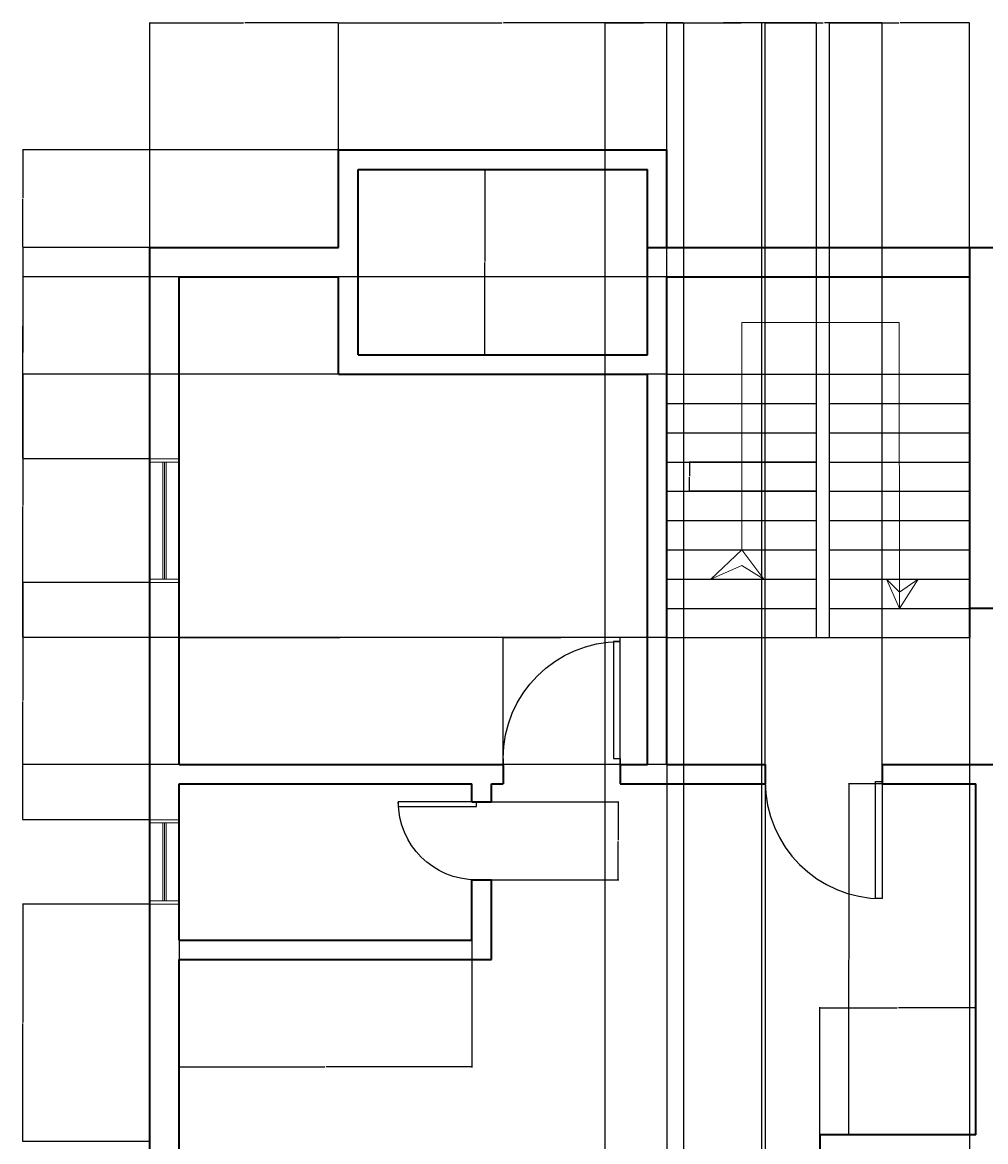
# Model space of a CAD drawing. Units: inches. Extents: x -7288 to -6705, y 7169 to 8028.
# Tile 4 of 5: x -7288 to -6992, y 7684 to 8028. Entities that reach past the tile are written whole.
import ezdxf

# ---------------------------------------------------------------- set-up
doc = ezdxf.new("R2010")
doc.units = ezdxf.units.IN
for name, color, linetype, lineweight in [('A-ANNO-DIMS', 2, 'Continuous', 18), ('A-ANNO-SYMB', 7, 'Continuous', 18), ('A-DOOR', 3, 'Continuous', 25), ('A-FLOR-STRS', 1, 'Continuous', 25), ('A-GLAZ', 2, 'Continuous', 18), ('A-WALL', 1, 'Continuous', 35)]:
    doc.layers.add(name, color=color, linetype=linetype, lineweight=lineweight)
doc.styles.get("Standard").update_dxf_attribs({"font": 'arial.ttf'})
doc.dimstyles.get("Standard").update_dxf_attribs({"dimtxt": 0.18, "dimasz": 0.18, "dimexe": 0.18, "dimexo": 0.0625, "dimgap": 0.09, "dimtad": 0, "dimtih": 1, "dimtoh": 1, "dimdec": 4, "dimzin": 0, "dimdsep": 46, "dimtxsty": 'Standard', "dimcen": 0.09, "dimadec": 0, "dimazin": 0, "dimtfac": 1, "dimtdec": 4, "dimtofl": 0, "dimtmove": 0, "dimatfit": 3, "dimfxl": 1, "dimtolj": 1, "dimtzin": 0, "dimarcsym": 0})

# ---------------------------------------------------------------- blocks, each defined once
blk = doc.blocks.new('*U8')
for p, q in [((0, 0), (0, -100)), ((750, 0), (750, -100))]:
    blk.add_line(p, q)
blk.add_lwpolyline([(0, 0), (0, 750), (43.75, 750), (43.75, 0)], close=True)
blk.add_arc((0, 0), 750, 0, 90)
blk = doc.blocks.new('WIN-36IN-WALL9')
for p, q in [((0, 38), (9, 38)), ((0, 37), (9, 37)), ((4, 1), (4, 37)), ((4.5, 1), (4.5, 37)), ((5, 1), (5, 37)), ((0, 1), (9, 1)), ((0, 0), (9, 0))]:
    blk.add_line(p, q)
blk = doc.blocks.new('WIN-24IN-WALL9')
for p, q in [((0, 26), (9, 26)), ((0, 25), (9, 25)), ((4, 1), (4, 25)), ((4.5, 1), (4.5, 25)), ((5, 1), (5, 25)), ((0, 1), (9, 1)), ((0, 0), (9, 0))]:
    blk.add_line(p, q)
blk = doc.blocks.new('*D95')
at = {"layer": 'A-ANNO-DIMS', "color": 0, "lineweight": -2, "transparency": 16777216}
for p, q in [((-7248.84, 7958.59), (-7248.84, 8027.74)), ((-7248.66, 8027.56), (-7220.06, 8027.56)), ((-7191.02, 8027.56), (-7219.62, 8027.56)), ((-7190.84, 7988.59), (-7190.84, 8027.74))]:
    blk.add_line(p, q, dxfattribs=at)
at = {"layer": 'A-ANNO-DIMS', "color": 0, "transparency": 16777216}
for points in [[(-7248.66, 8027.59), (-7248.66, 8027.53), (-7248.84, 8027.56)], [(-7191.02, 8027.59), (-7191.02, 8027.53), (-7190.84, 8027.56)]]:
    blk.add_solid(points, dxfattribs=at)
at = {"layer": 'Defpoints', "color": 0, "transparency": 16777216}
for p in [(-7190.84, 8027.56), (-7190.84, 7988.53), (-7248.84, 7958.53)]:
    blk.add_point(p, dxfattribs=at)
at = {"layer": 'A-ANNO-DIMS', "color": 0, "transparency": 16777216, "insert": (-7219.84, 8027.56), "char_height": 0.18, "attachment_point": 5}
blk.add_mtext('\\A1;58', dxfattribs=at)
blk = doc.blocks.new('*D96')
at = {"layer": 'A-ANNO-DIMS', "color": 0, "lineweight": -2, "transparency": 16777216}
for p, q in [((-7190.84, 7988.59), (-7190.84, 8027.74)), ((-7190.66, 8027.56), (-7140.6, 8027.56)), ((-7090.02, 8027.56), (-7140.08, 8027.56)), ((-7089.84, 7988.59), (-7089.84, 8027.74))]:
    blk.add_line(p, q, dxfattribs=at)
at = {"layer": 'A-ANNO-DIMS', "color": 0, "transparency": 16777216}
for points in [[(-7190.66, 8027.59), (-7190.66, 8027.53), (-7190.84, 8027.56)], [(-7090.02, 8027.59), (-7090.02, 8027.53), (-7089.84, 8027.56)]]:
    blk.add_solid(points, dxfattribs=at)
at = {"layer": 'Defpoints', "color": 0, "transparency": 16777216}
for p in [(-7089.84, 8027.56), (-7190.84, 7988.53), (-7089.84, 7988.53)]:
    blk.add_point(p, dxfattribs=at)
at = {"layer": 'A-ANNO-DIMS', "color": 0, "transparency": 16777216, "insert": (-7140.34, 8027.56), "char_height": 0.18, "attachment_point": 5}
blk.add_mtext('\\A1;101', dxfattribs=at)
blk = doc.blocks.new('*D99')
at = {"layer": 'A-ANNO-DIMS', "color": 0, "lineweight": -2, "transparency": 16777216}
for p, q in [((-7190.9, 7988.53), (-7288.05, 7988.53)), ((-7287.87, 7988.35), (-7287.87, 7973.71)), ((-7287.87, 7958.71), (-7287.87, 7973.35)), ((-7190.9, 7958.53), (-7288.05, 7958.53))]:
    blk.add_line(p, q, dxfattribs=at)
at = {"layer": 'A-ANNO-DIMS', "color": 0, "transparency": 16777216}
for points in [[(-7287.9, 7988.35), (-7287.84, 7988.35), (-7287.87, 7988.53)], [(-7287.9, 7958.71), (-7287.84, 7958.71), (-7287.87, 7958.53)]]:
    blk.add_solid(points, dxfattribs=at)
at = {"layer": 'Defpoints', "color": 0, "transparency": 16777216}
for p in [(-7287.87, 7988.53), (-7190.84, 7988.53), (-7190.84, 7958.53)]:
    blk.add_point(p, dxfattribs=at)
at = {"layer": 'A-ANNO-DIMS', "color": 0, "transparency": 16777216, "insert": (-7287.87, 7973.53), "char_height": 0.18, "attachment_point": 5}
blk.add_mtext('\\A1;30', dxfattribs=at)
blk = doc.blocks.new('*D103')
at = {"layer": 'A-ANNO-DIMS', "color": 0, "lineweight": -2, "transparency": 16777216}
for p, q in [((-7089.84, 7838.47), (-7089.84, 7169.32)), ((-6996.84, 7838.47), (-6996.84, 7169.32)), ((-7089.66, 7169.5), (-7043.56, 7169.5)), ((-6997.02, 7169.5), (-7043.12, 7169.5))]:
    blk.add_line(p, q, dxfattribs=at)
at = {"layer": 'A-ANNO-DIMS', "color": 0, "transparency": 16777216}
for points in [[(-7089.66, 7169.53), (-7089.66, 7169.47), (-7089.84, 7169.5)], [(-6997.02, 7169.53), (-6997.02, 7169.47), (-6996.84, 7169.5)]]:
    blk.add_solid(points, dxfattribs=at)
at = {"layer": 'Defpoints', "color": 0, "transparency": 16777216}
for p in [(-7089.84, 7838.53), (-6996.84, 7838.53), (-6996.84, 7169.5)]:
    blk.add_point(p, dxfattribs=at)
at = {"layer": 'A-ANNO-DIMS', "color": 0, "transparency": 16777216, "insert": (-7043.34, 7169.5), "char_height": 0.18, "attachment_point": 5}
blk.add_mtext('\\A1;93', dxfattribs=at)
blk = doc.blocks.new('*D106')
at = {"layer": 'A-ANNO-DIMS', "color": 0, "lineweight": -2, "transparency": 16777216}
for p, q in [((-7089.9, 7919.53), (-7288.05, 7919.53)), ((-7287.87, 7919.35), (-7287.87, 7879.21)), ((-7287.87, 7838.71), (-7287.87, 7878.85)), ((-7089.9, 7838.53), (-7288.05, 7838.53))]:
    blk.add_line(p, q, dxfattribs=at)
at = {"layer": 'A-ANNO-DIMS', "color": 0, "transparency": 16777216}
for points in [[(-7287.9, 7919.35), (-7287.84, 7919.35), (-7287.87, 7919.53)], [(-7287.9, 7838.71), (-7287.84, 7838.71), (-7287.87, 7838.53)]]:
    blk.add_solid(points, dxfattribs=at)
at = {"layer": 'Defpoints', "color": 0, "transparency": 16777216}
for p in [(-7287.87, 7919.53), (-7089.84, 7919.53), (-7089.84, 7838.53)]:
    blk.add_point(p, dxfattribs=at)
at = {"layer": 'A-ANNO-DIMS', "color": 0, "transparency": 16777216, "insert": (-7287.87, 7879.03), "char_height": 0.18, "attachment_point": 5}
blk.add_mtext('\\A1;81', dxfattribs=at)
blk = doc.blocks.new('*D107')
at = {"layer": 'A-ANNO-DIMS', "color": 0, "lineweight": -2, "transparency": 16777216}
for p, q in [((-7089.9, 7949.53), (-7288.05, 7949.53)), ((-7287.87, 7949.35), (-7287.87, 7934.71)), ((-7287.87, 7919.71), (-7287.87, 7934.35)), ((-7089.9, 7919.53), (-7288.05, 7919.53))]:
    blk.add_line(p, q, dxfattribs=at)
at = {"layer": 'A-ANNO-DIMS', "color": 0, "transparency": 16777216}
for points in [[(-7287.9, 7949.35), (-7287.84, 7949.35), (-7287.87, 7949.53)], [(-7287.9, 7919.71), (-7287.84, 7919.71), (-7287.87, 7919.53)]]:
    blk.add_solid(points, dxfattribs=at)
at = {"layer": 'Defpoints', "color": 0, "transparency": 16777216}
for p in [(-7287.87, 7949.53), (-7089.84, 7949.53), (-7089.84, 7919.53)]:
    blk.add_point(p, dxfattribs=at)
at = {"layer": 'A-ANNO-DIMS', "color": 0, "transparency": 16777216, "insert": (-7287.87, 7934.53), "char_height": 0.18, "attachment_point": 5}
blk.add_mtext('\\A1;30', dxfattribs=at)
blk = doc.blocks.new('*D108')
at = {"layer": 'A-ANNO-DIMS', "color": 0, "lineweight": -2, "transparency": 16777216}
for p, q in [((-7089.9, 7838.53), (-7288.05, 7838.53)), ((-7287.87, 7838.35), (-7287.87, 7819.21)), ((-7287.87, 7799.71), (-7287.87, 7818.85)), ((-7089.9, 7799.53), (-7288.05, 7799.53))]:
    blk.add_line(p, q, dxfattribs=at)
at = {"layer": 'A-ANNO-DIMS', "color": 0, "transparency": 16777216}
for points in [[(-7287.9, 7838.35), (-7287.84, 7838.35), (-7287.87, 7838.53)], [(-7287.9, 7799.71), (-7287.84, 7799.71), (-7287.87, 7799.53)]]:
    blk.add_solid(points, dxfattribs=at)
at = {"layer": 'Defpoints', "color": 0, "transparency": 16777216}
for p in [(-7287.87, 7838.53), (-7089.84, 7838.53), (-7089.84, 7799.53)]:
    blk.add_point(p, dxfattribs=at)
at = {"layer": 'A-ANNO-DIMS', "color": 0, "transparency": 16777216, "insert": (-7287.87, 7819.03), "char_height": 0.18, "attachment_point": 5}
blk.add_mtext('\\A1;39', dxfattribs=at)
blk = doc.blocks.new('*D110')
at = {"layer": 'A-ANNO-DIMS', "color": 0, "lineweight": -2, "transparency": 16777216}
for p, q in [((-7089.84, 7838.59), (-7089.84, 8027.74)), ((-7089.66, 8027.56), (-7067.06, 8027.56)), ((-7044.02, 8027.56), (-7066.62, 8027.56)), ((-7043.84, 7838.59), (-7043.84, 8027.74))]:
    blk.add_line(p, q, dxfattribs=at)
at = {"layer": 'A-ANNO-DIMS', "color": 0, "transparency": 16777216}
for points in [[(-7089.66, 8027.59), (-7089.66, 8027.53), (-7089.84, 8027.56)], [(-7044.02, 8027.59), (-7044.02, 8027.53), (-7043.84, 8027.56)]]:
    blk.add_solid(points, dxfattribs=at)
at = {"layer": 'Defpoints', "color": 0, "transparency": 16777216}
for p in [(-7043.84, 8027.56), (-7089.84, 7838.53), (-7043.84, 7838.53)]:
    blk.add_point(p, dxfattribs=at)
at = {"layer": 'A-ANNO-DIMS', "color": 0, "transparency": 16777216, "insert": (-7066.84, 8027.56), "char_height": 0.18, "attachment_point": 5}
blk.add_mtext('\\A1;46', dxfattribs=at)
blk = doc.blocks.new('*D111')
at = {"layer": 'A-ANNO-DIMS', "color": 0, "lineweight": -2, "transparency": 16777216}
for p, q in [((-7039.84, 7919.59), (-7039.84, 8027.74)), ((-7039.66, 8027.56), (-7018.56, 8027.56)), ((-6997.02, 8027.56), (-7018.12, 8027.56)), ((-6996.84, 7919.59), (-6996.84, 8027.74))]:
    blk.add_line(p, q, dxfattribs=at)
at = {"layer": 'A-ANNO-DIMS', "color": 0, "transparency": 16777216}
for points in [[(-7039.66, 8027.59), (-7039.66, 8027.53), (-7039.84, 8027.56)], [(-6997.02, 8027.59), (-6997.02, 8027.53), (-6996.84, 8027.56)]]:
    blk.add_solid(points, dxfattribs=at)
at = {"layer": 'Defpoints', "color": 0, "transparency": 16777216}
for p in [(-6996.84, 8027.56), (-7039.84, 7919.53), (-6996.84, 7919.53)]:
    blk.add_point(p, dxfattribs=at)
at = {"layer": 'A-ANNO-DIMS', "color": 0, "transparency": 16777216, "insert": (-7018.34, 8027.56), "char_height": 0.18, "attachment_point": 5}
blk.add_mtext('\\A1;43', dxfattribs=at)
blk = doc.blocks.new('*D112')
at = {"layer": 'A-ANNO-DIMS', "color": 0, "lineweight": -2, "transparency": 16777216}
for p, q in [((-7043.9, 7892.53), (-7083.05, 7892.53)), ((-7082.87, 7892.35), (-7082.87, 7888.21)), ((-7082.87, 7883.71), (-7082.87, 7887.85)), ((-7043.9, 7883.53), (-7083.05, 7883.53))]:
    blk.add_line(p, q, dxfattribs=at)
at = {"layer": 'A-ANNO-DIMS', "color": 0, "transparency": 16777216}
for points in [[(-7082.9, 7892.35), (-7082.84, 7892.35), (-7082.87, 7892.53)], [(-7082.9, 7883.71), (-7082.84, 7883.71), (-7082.87, 7883.53)]]:
    blk.add_solid(points, dxfattribs=at)
at = {"layer": 'Defpoints', "color": 0, "transparency": 16777216}
for p in [(-7082.87, 7892.53), (-7043.84, 7892.53), (-7043.84, 7883.53)]:
    blk.add_point(p, dxfattribs=at)
at = {"layer": 'A-ANNO-DIMS', "color": 0, "transparency": 16777216, "insert": (-7082.87, 7888.03), "char_height": 0.18, "attachment_point": 5}
blk.add_mtext('\\A1;9', dxfattribs=at)
blk = doc.blocks.new('*D118')
at = {"layer": 'A-ANNO-DIMS', "color": 0, "lineweight": -2, "transparency": 16777216}
for p, q in [((-7059.61, 7799.59), (-7059.61, 8027.74)), ((-7059.43, 8027.56), (-7041.83, 8027.56)), ((-7023.79, 8027.56), (-7041.39, 8027.56)), ((-7023.61, 7799.59), (-7023.61, 8027.74))]:
    blk.add_line(p, q, dxfattribs=at)
at = {"layer": 'A-ANNO-DIMS', "color": 0, "transparency": 16777216}
for points in [[(-7059.43, 8027.59), (-7059.43, 8027.53), (-7059.61, 8027.56)], [(-7023.79, 8027.59), (-7023.79, 8027.53), (-7023.61, 8027.56)]]:
    blk.add_solid(points, dxfattribs=at)
at = {"layer": 'Defpoints', "color": 0, "transparency": 16777216}
for p in [(-7023.61, 8027.56), (-7059.61, 7799.53), (-7023.61, 7799.53)]:
    blk.add_point(p, dxfattribs=at)
at = {"layer": 'A-ANNO-DIMS', "color": 0, "transparency": 16777216, "insert": (-7041.61, 8027.56), "char_height": 0.18, "attachment_point": 5}
blk.add_mtext('\\A1;36', dxfattribs=at)
blk = doc.blocks.new('*D119')
at = {"layer": 'A-ANNO-DIMS', "color": 0, "lineweight": -2, "transparency": 16777216}
for p, q in [((-7089.84, 7799.47), (-7089.84, 7169.32)), ((-7059.61, 7799.47), (-7059.61, 7169.32)), ((-7089.66, 7169.5), (-7075.12, 7169.5)), ((-7059.79, 7169.5), (-7074.33, 7169.5))]:
    blk.add_line(p, q, dxfattribs=at)
at = {"layer": 'A-ANNO-DIMS', "color": 0, "transparency": 16777216}
for points in [[(-7089.66, 7169.53), (-7089.66, 7169.47), (-7089.84, 7169.5)], [(-7059.79, 7169.53), (-7059.79, 7169.47), (-7059.61, 7169.5)]]:
    blk.add_solid(points, dxfattribs=at)
at = {"layer": 'Defpoints', "color": 0, "transparency": 16777216}
for p in [(-7089.84, 7799.53), (-7059.61, 7799.53), (-7059.61, 7169.5)]:
    blk.add_point(p, dxfattribs=at)
at = {"layer": 'A-ANNO-DIMS', "color": 0, "transparency": 16777216, "insert": (-7074.72, 7169.5), "char_height": 0.18, "attachment_point": 5}
blk.add_mtext('\\A1;30.23', dxfattribs=at)
blk = doc.blocks.new('*D122')
at = {"layer": 'A-ANNO-DIMS', "color": 0, "lineweight": -2, "transparency": 16777216}
for p, q in [((-7239.84, 7799.59), (-7239.84, 7838.74)), ((-7239.66, 7838.56), (-7190.42, 7838.56)), ((-7140.4, 7838.56), (-7189.64, 7838.56)), ((-7140.22, 7799.59), (-7140.22, 7838.74))]:
    blk.add_line(p, q, dxfattribs=at)
at = {"layer": 'A-ANNO-DIMS', "color": 0, "transparency": 16777216}
for points in [[(-7239.66, 7838.59), (-7239.66, 7838.53), (-7239.84, 7838.56)], [(-7140.4, 7838.59), (-7140.4, 7838.53), (-7140.22, 7838.56)]]:
    blk.add_solid(points, dxfattribs=at)
at = {"layer": 'Defpoints', "color": 0, "transparency": 16777216}
for p in [(-7140.22, 7838.56), (-7239.84, 7799.53), (-7140.22, 7799.53)]:
    blk.add_point(p, dxfattribs=at)
at = {"layer": 'A-ANNO-DIMS', "color": 0, "transparency": 16777216, "insert": (-7190.03, 7838.56), "char_height": 0.18, "attachment_point": 5}
blk.add_mtext('\\A1;99.62', dxfattribs=at)
blk = doc.blocks.new('*D123')
at = {"layer": 'A-ANNO-DIMS', "color": 0, "lineweight": -2, "transparency": 16777216}
for p, q in [((-7140.22, 7799.59), (-7140.22, 7838.74)), ((-7140.04, 7838.56), (-7122.44, 7838.56)), ((-7104.4, 7838.56), (-7122, 7838.56)), ((-7104.22, 7799.59), (-7104.22, 7838.74))]:
    blk.add_line(p, q, dxfattribs=at)
at = {"layer": 'A-ANNO-DIMS', "color": 0, "transparency": 16777216}
for points in [[(-7140.04, 7838.59), (-7140.04, 7838.53), (-7140.22, 7838.56)], [(-7104.4, 7838.59), (-7104.4, 7838.53), (-7104.22, 7838.56)]]:
    blk.add_solid(points, dxfattribs=at)
at = {"layer": 'Defpoints', "color": 0, "transparency": 16777216}
for p in [(-7104.22, 7838.56), (-7140.22, 7799.53), (-7104.22, 7799.53)]:
    blk.add_point(p, dxfattribs=at)
at = {"layer": 'A-ANNO-DIMS', "color": 0, "transparency": 16777216, "insert": (-7122.22, 7838.56), "char_height": 0.18, "attachment_point": 5}
blk.add_mtext('\\A1;36', dxfattribs=at)
blk = doc.blocks.new('*D126')
at = {"layer": 'A-ANNO-DIMS', "color": 0, "lineweight": -2, "transparency": 16777216}
for p, q in [((-7184.78, 7982.53), (-7145.63, 7982.53)), ((-7145.81, 7982.35), (-7145.81, 7954.21)), ((-7145.81, 7925.71), (-7145.81, 7953.85)), ((-7184.78, 7925.53), (-7145.63, 7925.53))]:
    blk.add_line(p, q, dxfattribs=at)
at = {"layer": 'A-ANNO-DIMS', "color": 0, "transparency": 16777216}
for points in [[(-7145.84, 7982.35), (-7145.78, 7982.35), (-7145.81, 7982.53)], [(-7145.84, 7925.71), (-7145.78, 7925.71), (-7145.81, 7925.53)]]:
    blk.add_solid(points, dxfattribs=at)
at = {"layer": 'Defpoints', "color": 0, "transparency": 16777216}
for p in [(-7184.84, 7982.53), (-7184.84, 7925.53), (-7145.81, 7925.53)]:
    blk.add_point(p, dxfattribs=at)
at = {"layer": 'A-ANNO-DIMS', "color": 0, "transparency": 16777216, "insert": (-7145.81, 7954.03), "char_height": 0.18, "attachment_point": 5}
blk.add_mtext('\\A1;57', dxfattribs=at)
blk = doc.blocks.new('*D127')
at = {"layer": 'A-ANNO-DIMS', "color": 0, "lineweight": -2, "transparency": 16777216}
for p, q in [((-7239.84, 7745.47), (-7239.84, 7706.32)), ((-7149.84, 7745.47), (-7149.84, 7706.32)), ((-7239.66, 7706.5), (-7195.06, 7706.5)), ((-7150.02, 7706.5), (-7194.62, 7706.5))]:
    blk.add_line(p, q, dxfattribs=at)
at = {"layer": 'A-ANNO-DIMS', "color": 0, "transparency": 16777216}
for points in [[(-7239.66, 7706.53), (-7239.66, 7706.47), (-7239.84, 7706.5)], [(-7150.02, 7706.53), (-7150.02, 7706.47), (-7149.84, 7706.5)]]:
    blk.add_solid(points, dxfattribs=at)
at = {"layer": 'Defpoints', "color": 0, "transparency": 16777216}
for p in [(-7239.84, 7745.53), (-7149.84, 7745.53), (-7239.84, 7706.5)]:
    blk.add_point(p, dxfattribs=at)
at = {"layer": 'A-ANNO-DIMS', "color": 0, "transparency": 16777216, "insert": (-7194.84, 7706.5), "char_height": 0.18, "attachment_point": 5}
blk.add_mtext('\\A1;90', dxfattribs=at)
blk = doc.blocks.new('*D129')
at = {"layer": 'A-ANNO-DIMS', "color": 0, "lineweight": -2, "transparency": 16777216}
for p, q in [((-7143.78, 7788.02), (-7104.63, 7788.02)), ((-7104.81, 7787.84), (-7104.81, 7776.2)), ((-7104.81, 7764.2), (-7104.81, 7775.84)), ((-7143.78, 7764.02), (-7104.63, 7764.02))]:
    blk.add_line(p, q, dxfattribs=at)
at = {"layer": 'A-ANNO-DIMS', "color": 0, "transparency": 16777216}
for points in [[(-7104.84, 7787.84), (-7104.78, 7787.84), (-7104.81, 7788.02)], [(-7104.84, 7764.2), (-7104.78, 7764.2), (-7104.81, 7764.02)]]:
    blk.add_solid(points, dxfattribs=at)
at = {"layer": 'Defpoints', "color": 0, "transparency": 16777216}
for p in [(-7143.84, 7788.02), (-7143.84, 7764.02), (-7104.81, 7764.02)]:
    blk.add_point(p, dxfattribs=at)
at = {"layer": 'A-ANNO-DIMS', "color": 0, "transparency": 16777216, "insert": (-7104.81, 7776.02), "char_height": 0.18, "attachment_point": 5}
blk.add_mtext('\\A1;24', dxfattribs=at)
blk = doc.blocks.new('*D134')
at = {"layer": 'A-ANNO-DIMS', "color": 0, "lineweight": -2, "transparency": 16777216}
for p, q in [((-7042.84, 7685.7), (-7042.84, 7724.85)), ((-7042.66, 7724.67), (-7019.06, 7724.67)), ((-6995.02, 7724.67), (-7018.62, 7724.67)), ((-6994.84, 7685.7), (-6994.84, 7724.85))]:
    blk.add_line(p, q, dxfattribs=at)
at = {"layer": 'A-ANNO-DIMS', "color": 0, "transparency": 16777216}
for points in [[(-7042.66, 7724.7), (-7042.66, 7724.64), (-7042.84, 7724.67)], [(-6995.02, 7724.7), (-6995.02, 7724.64), (-6994.84, 7724.67)]]:
    blk.add_solid(points, dxfattribs=at)
at = {"layer": 'Defpoints', "color": 0, "transparency": 16777216}
for p in [(-6994.84, 7724.67), (-7042.84, 7685.64), (-6994.84, 7685.64)]:
    blk.add_point(p, dxfattribs=at)
at = {"layer": 'A-ANNO-DIMS', "color": 0, "transparency": 16777216, "insert": (-7018.84, 7724.67), "char_height": 0.18, "attachment_point": 5}
blk.add_mtext('\\A1;48', dxfattribs=at)
blk = doc.blocks.new('*D135')
at = {"layer": 'A-ANNO-DIMS', "color": 0, "lineweight": -2, "transparency": 16777216}
for p, q in [((-6994.9, 7793.53), (-7034.05, 7793.53)), ((-7033.87, 7793.35), (-7033.87, 7739.77)), ((-7033.87, 7685.82), (-7033.87, 7739.4)), ((-6994.9, 7685.64), (-7034.05, 7685.64))]:
    blk.add_line(p, q, dxfattribs=at)
at = {"layer": 'A-ANNO-DIMS', "color": 0, "transparency": 16777216}
for points in [[(-7033.9, 7793.35), (-7033.84, 7793.35), (-7033.87, 7793.53)], [(-7033.9, 7685.82), (-7033.84, 7685.82), (-7033.87, 7685.64)]]:
    blk.add_solid(points, dxfattribs=at)
at = {"layer": 'Defpoints', "color": 0, "transparency": 16777216}
for p in [(-7033.87, 7793.53), (-6994.84, 7793.53), (-6994.84, 7685.64)]:
    blk.add_point(p, dxfattribs=at)
at = {"layer": 'A-ANNO-DIMS', "color": 0, "transparency": 16777216, "insert": (-7033.87, 7739.59), "char_height": 0.18, "attachment_point": 5}
blk.add_mtext('\\A1;107.9', dxfattribs=at)
blk = doc.blocks.new('*D150')
at = {"layer": 'A-ANNO-DIMS', "color": 0, "lineweight": -2, "transparency": 16777216}
for p, q in [((-7248.9, 7756.53), (-7288.05, 7756.53)), ((-7287.87, 7756.35), (-7287.87, 7720.21)), ((-7287.87, 7683.71), (-7287.87, 7719.85)), ((-7248.9, 7683.53), (-7288.05, 7683.53))]:
    blk.add_line(p, q, dxfattribs=at)
at = {"layer": 'A-ANNO-DIMS', "color": 0, "transparency": 16777216}
for points in [[(-7287.9, 7756.35), (-7287.84, 7756.35), (-7287.87, 7756.53)], [(-7287.9, 7683.71), (-7287.84, 7683.71), (-7287.87, 7683.53)]]:
    blk.add_solid(points, dxfattribs=at)
at = {"layer": 'Defpoints', "color": 0, "transparency": 16777216}
for p in [(-7287.87, 7756.53), (-7248.84, 7756.53), (-7248.84, 7683.53)]:
    blk.add_point(p, dxfattribs=at)
at = {"layer": 'A-ANNO-DIMS', "color": 0, "transparency": 16777216, "insert": (-7287.87, 7720.03), "char_height": 0.18, "attachment_point": 5}
blk.add_mtext('\\A1;73', dxfattribs=at)
blk = doc.blocks.new('*D151')
at = {"layer": 'A-ANNO-DIMS', "color": 0, "lineweight": -2, "transparency": 16777216}
for p, q in [((-7248.9, 7855.53), (-7288.05, 7855.53)), ((-7287.87, 7855.35), (-7287.87, 7819.21)), ((-7287.87, 7782.71), (-7287.87, 7818.85)), ((-7248.9, 7782.53), (-7288.05, 7782.53))]:
    blk.add_line(p, q, dxfattribs=at)
at = {"layer": 'A-ANNO-DIMS', "color": 0, "transparency": 16777216}
for points in [[(-7287.9, 7855.35), (-7287.84, 7855.35), (-7287.87, 7855.53)], [(-7287.9, 7782.71), (-7287.84, 7782.71), (-7287.87, 7782.53)]]:
    blk.add_solid(points, dxfattribs=at)
at = {"layer": 'Defpoints', "color": 0, "transparency": 16777216}
for p in [(-7287.87, 7855.53), (-7248.84, 7855.53), (-7248.84, 7782.53)]:
    blk.add_point(p, dxfattribs=at)
at = {"layer": 'A-ANNO-DIMS', "color": 0, "transparency": 16777216, "insert": (-7287.87, 7819.03), "char_height": 0.18, "attachment_point": 5}
blk.add_mtext('\\A1;73', dxfattribs=at)
blk = doc.blocks.new('*D152')
at = {"layer": 'A-ANNO-DIMS', "color": 0, "lineweight": -2, "transparency": 16777216}
for p, q in [((-7248.9, 7958.53), (-7288.05, 7958.53)), ((-7287.87, 7958.35), (-7287.87, 7926.21)), ((-7287.87, 7893.71), (-7287.87, 7925.85)), ((-7248.9, 7893.53), (-7288.05, 7893.53))]:
    blk.add_line(p, q, dxfattribs=at)
at = {"layer": 'A-ANNO-DIMS', "color": 0, "transparency": 16777216}
for points in [[(-7287.9, 7958.35), (-7287.84, 7958.35), (-7287.87, 7958.53)], [(-7287.9, 7893.71), (-7287.84, 7893.71), (-7287.87, 7893.53)]]:
    blk.add_solid(points, dxfattribs=at)
at = {"layer": 'Defpoints', "color": 0, "transparency": 16777216}
for p in [(-7287.87, 7958.53), (-7248.84, 7958.53), (-7248.84, 7893.53)]:
    blk.add_point(p, dxfattribs=at)
at = {"layer": 'A-ANNO-DIMS', "color": 0, "transparency": 16777216, "insert": (-7287.87, 7926.03), "char_height": 0.18, "attachment_point": 5}
blk.add_mtext('\\A1;65', dxfattribs=at)
blk = doc.blocks.new('*D156')
at = {"layer": 'A-ANNO-DIMS', "color": 0, "lineweight": -2, "transparency": 16777216}
for p, q in [((-7084.64, 7347.59), (-7084.64, 8027.74)), ((-7084.46, 8027.56), (-7072.86, 8027.56)), ((-7060.82, 8027.56), (-7072.42, 8027.56)), ((-7060.64, 7347.59), (-7060.64, 8027.74))]:
    blk.add_line(p, q, dxfattribs=at)
at = {"layer": 'A-ANNO-DIMS', "color": 0, "transparency": 16777216}
for points in [[(-7084.46, 8027.59), (-7084.46, 8027.53), (-7084.64, 8027.56)], [(-7060.82, 8027.59), (-7060.82, 8027.53), (-7060.64, 8027.56)]]:
    blk.add_solid(points, dxfattribs=at)
at = {"layer": 'Defpoints', "color": 0, "transparency": 16777216}
for p in [(-7060.64, 8027.56), (-7084.64, 7347.53), (-7060.64, 7347.53)]:
    blk.add_point(p, dxfattribs=at)
at = {"layer": 'A-ANNO-DIMS', "color": 0, "transparency": 16777216, "insert": (-7072.64, 8027.56), "char_height": 0.18, "attachment_point": 5}
blk.add_mtext('\\A1;24', dxfattribs=at)
blk = doc.blocks.new('*D157')
at = {"layer": 'A-ANNO-DIMS', "color": 0, "lineweight": -2, "transparency": 16777216}
for p, q in [((-7108.84, 7347.59), (-7108.84, 8027.74)), ((-7108.66, 8027.56), (-7097.07, 8027.56)), ((-7084.82, 8027.56), (-7096.42, 8027.56)), ((-7084.64, 7347.59), (-7084.64, 8027.74))]:
    blk.add_line(p, q, dxfattribs=at)
at = {"layer": 'A-ANNO-DIMS', "color": 0, "transparency": 16777216}
for points in [[(-7108.66, 8027.59), (-7108.66, 8027.53), (-7108.84, 8027.56)], [(-7084.82, 8027.59), (-7084.82, 8027.53), (-7084.64, 8027.56)]]:
    blk.add_solid(points, dxfattribs=at)
at = {"layer": 'Defpoints', "color": 0, "transparency": 16777216}
for p in [(-7084.64, 8027.56), (-7108.84, 7347.53), (-7084.64, 7347.53)]:
    blk.add_point(p, dxfattribs=at)
at = {"layer": 'A-ANNO-DIMS', "color": 0, "transparency": 16777216, "insert": (-7096.74, 8027.56), "char_height": 0.18, "attachment_point": 5}
blk.add_mtext('\\A1;24.2', dxfattribs=at)

msp = doc.modelspace()

# ---------------------------------------------------------------- linework, layer by layer
at = {"layer": 'A-ANNO-SYMB'}
for p, q in [((-7066.8398, 7865.5311), (-7066.8398, 7935.4325)), ((-7066.8398, 7935.4325), (-7018.4183, 7935.4325)), ((-7018.4183, 7935.4325), (-7018.3398, 7847.5311)), ((-7066.8398, 7865.5311), (-7076.3422, 7856.5311)), ((-7060.0902, 7856.5311), (-7066.8398, 7865.5311)), ((-7076.3422, 7856.5311), (-7066.8398, 7860.6787)), ((-7066.8398, 7860.6787), (-7060.0902, 7856.5311)), ((-7076.3422, 7856.5311), (-7066.8398, 7856.5311)), ((-7076.3422, 7856.5311), (-7067.18, 7856.5311)), ((-7067.18, 7856.5311), (-7060.0902, 7856.5311)), ((-7066.8398, 7856.5311), (-7060.0902, 7856.5311)), ((-7018.3442, 7852.4713), (-7022.3015, 7856.5311)), ((-7022.3015, 7856.5311), (-7018.3398, 7847.5311)), ((-7012.5731, 7856.5311), (-7018.3442, 7852.4713)), ((-7018.3398, 7847.5311), (-7012.5731, 7856.5311))]:
    msp.add_line(p, q, dxfattribs=at)
at = {"layer": 'A-FLOR-STRS'}
for p, q in [((-7089.8398, 7919.5311), (-6996.8398, 7919.5311)), ((-7043.8398, 7838.5311), (-7043.8398, 7919.5311)), ((-7039.8398, 7838.5311), (-7039.8398, 7919.5311)), ((-7089.8398, 7910.5311), (-7043.8398, 7910.5311)), ((-7039.8398, 7910.5311), (-6996.8398, 7910.5311)), ((-7089.8398, 7901.5311), (-7043.8398, 7901.5311)), ((-7039.8398, 7901.5311), (-6996.8398, 7901.5311)), ((-7089.8398, 7892.5311), (-7043.8398, 7892.5311)), ((-7039.8398, 7892.5311), (-6996.8398, 7892.5311)), ((-7089.8398, 7883.5311), (-7043.8398, 7883.5311)), ((-7039.8398, 7883.5311), (-6996.8398, 7883.5311)), ((-7089.8398, 7874.5311), (-7043.8398, 7874.5311)), ((-7039.8398, 7874.5311), (-6996.8398, 7874.5311)), ((-7089.8398, 7865.5311), (-7043.8398, 7865.5311)), ((-7039.8398, 7865.5311), (-6996.8398, 7865.5311)), ((-7089.8398, 7856.5311), (-7043.8398, 7856.5311)), ((-7039.8398, 7856.5311), (-6996.8398, 7856.5311)), ((-7089.8398, 7847.5311), (-7043.8398, 7847.5311)), ((-7039.8398, 7847.5311), (-6996.8398, 7847.5311)), ((-7089.8398, 7838.5311), (-6996.8398, 7838.5311))]:
    msp.add_line(p, q, dxfattribs=at)
at = {"layer": 'A-WALL'}
for p, q in [((-7190.8398, 7988.5311), (-7089.8398, 7988.5311)), ((-7190.8398, 7958.5311), (-7190.8398, 7988.5311)), ((-7089.8398, 7958.5311), (-7089.8398, 7988.5311)), ((-7184.8398, 7982.5311), (-7095.8398, 7982.5311)), ((-7184.8398, 7925.5311), (-7184.8398, 7982.5311)), ((-7095.8398, 7925.5311), (-7095.8398, 7982.5311)), ((-7248.8398, 7958.5311), (-7190.8398, 7958.5311)), ((-7248.8398, 7208.5311), (-7248.8398, 7958.5311)), ((-7095.8398, 7958.5311), (-6897.8398, 7958.5311)), ((-6996.8398, 7958.5311), (-6996.8398, 7838.5311)), ((-7239.8398, 7949.5311), (-7190.8398, 7949.5311)), ((-7239.8398, 7799.5311), (-7239.8398, 7949.5311)), ((-7190.8398, 7919.5311), (-7190.8398, 7949.5311)), ((-7089.8398, 7949.5311), (-6996.8398, 7949.5311)), ((-7089.8398, 7799.5311), (-7089.8398, 7949.5311)), ((-7184.8398, 7925.5311), (-7095.8398, 7925.5311)), ((-7190.8398, 7919.5311), (-7095.8398, 7919.5311)), ((-7095.8398, 7799.5311), (-7095.8398, 7919.5311)), ((-6987.8398, 7847.5311), (-6996.8398, 7847.5311)), ((-7239.8398, 7799.5311), (-7140.2215, 7799.5311)), ((-7140.2215, 7799.5311), (-7140.2215, 7793.5311)), ((-7104.2215, 7799.5311), (-7104.2215, 7793.5311)), ((-7104.2215, 7799.5311), (-7095.8398, 7799.5311)), ((-7089.8398, 7799.5311), (-7059.607, 7799.5311)), ((-7059.607, 7799.5311), (-7059.607, 7793.5311)), ((-7023.607, 7799.5311), (-7023.607, 7793.5311)), ((-7023.607, 7799.5311), (-6967.0693, 7799.5311)), ((-7239.8398, 7793.5311), (-7149.8398, 7793.5311)), ((-7239.8398, 7745.5311), (-7239.8398, 7793.5311)), ((-7149.8398, 7788.022), (-7149.8398, 7793.5311)), ((-7143.8398, 7793.5311), (-7140.2215, 7793.5311)), ((-7143.8398, 7788.022), (-7143.8398, 7793.5311)), ((-7104.2215, 7793.5311), (-7059.607, 7793.5311)), ((-7023.607, 7793.5311), (-6994.8398, 7793.5311)), ((-6994.8398, 7685.639), (-6994.8398, 7793.5311)), ((-7149.8398, 7788.022), (-7143.8398, 7788.022)), ((-7149.8398, 7745.5311), (-7149.8398, 7764.022)), ((-7149.8398, 7764.022), (-7143.8398, 7764.022)), ((-7143.8398, 7739.5311), (-7143.8398, 7764.022)), ((-7239.8398, 7745.5311), (-7149.8398, 7745.5311)), ((-7239.8398, 7745.5311), (-7149.8398, 7745.5311)), ((-7239.8398, 7739.5311), (-7143.8398, 7739.5311)), ((-7239.8398, 7739.5311), (-7143.8398, 7739.5311)), ((-7239.8398, 7589.5311), (-7239.8398, 7739.5311)), ((-6994.8398, 7685.639), (-7042.8398, 7685.639)), ((-7042.8398, 7685.639), (-7042.8398, 7679.639))]:
    msp.add_line(p, q, dxfattribs=at)

# ---------------------------------------------------------------- block references
at = {"layer": 'A-DOOR', "xscale": -0.0479999999999998, "yscale": 0.0479999999999998, "zscale": 0.0479999999999998}
msp.add_blockref('*U8', (-7104.2215, 7801.3311), dxfattribs=at)
at = {"layer": 'A-DOOR'}
for p, xscale, yscale, zscale, rotation in [((-7023.607, 7794.2499), 0.0479999999999998, 0.0479999999999998, 0.0479999999999998, 180), ((-7148.4398, 7788.022), -0.0320000000000005, 0.0320000000000005, 0.0320000000000005, 90)]:
    msp.add_blockref('*U8', p, dxfattribs=dict(at, xscale=xscale, yscale=yscale, zscale=zscale, rotation=rotation))
at = {"layer": 'A-GLAZ', "rotation": 180}
msp.add_blockref('WIN-36IN-WALL9', (-7239.8398, 7893.5311), dxfattribs=at)
at = {"layer": 'A-GLAZ'}
msp.add_blockref('WIN-24IN-WALL9', (-7248.8398, 7756.5311), dxfattribs=at)

# ---------------------------------------------------------------- dimensions: what is measured, and where the dimension line sits
at = {"layer": 'A-ANNO-DIMS'}
for base, p1, p2, override, picture, middle in [((-7190.8398, 8027.5611), (-7248.8398, 7958.5311), (-7190.8398, 7988.5311), {"dimdec": 0, "dimlfac": 1, "dimrnd": 0, "dimzin": 0, "dimdsep": 46, "dimlunit": 2}, '*D95', (-7219.8398, 8027.5611)), ((-7089.8398, 8027.5611), (-7190.8398, 7988.5311), (-7089.8398, 7988.5311), {"dimdec": 0, "dimlfac": 1, "dimrnd": 0, "dimzin": 0, "dimdsep": 46, "dimlunit": 2}, '*D96', (-7140.3398, 8027.5611)), ((-7084.6414, 8027.5611), (-7108.8398, 7347.5311), (-7084.6414, 7347.5311), {"dimdec": 1, "dimlfac": 1, "dimrnd": 0, "dimzin": 0, "dimdsep": 46, "dimlunit": 2}, '*D157', (-7096.7406, 8027.5611)), ((-7043.8398, 8027.5611), (-7089.8398, 7838.5311), (-7043.8398, 7838.5311), {"dimdec": 0, "dimlfac": 1, "dimrnd": 0, "dimzin": 0, "dimdsep": 46, "dimlunit": 2}, '*D110', (-7066.8398, 8027.5611)), ((-7060.6414, 8027.5611), (-7084.6414, 7347.5311), (-7060.6414, 7347.5311), {"dimdec": 0, "dimlfac": 1, "dimrnd": 0, "dimzin": 0, "dimdsep": 46, "dimlunit": 2}, '*D156', (-7072.6414, 8027.5611)), ((-7023.607, 8027.5611), (-7059.607, 7799.5311), (-7023.607, 7799.5311), {"dimdec": 0, "dimlfac": 1, "dimrnd": 0, "dimzin": 0, "dimdsep": 46, "dimlunit": 2}, '*D118', (-7041.607, 8027.5611)), ((-6996.8398, 8027.5611), (-7039.8398, 7919.5311), (-6996.8398, 7919.5311), {"dimdec": 0, "dimlfac": 1, "dimrnd": 0, "dimzin": 0, "dimdsep": 46, "dimlunit": 2}, '*D111', (-7018.3398, 8027.5611)), ((-7140.2215, 7838.5611), (-7239.8398, 7799.5311), (-7140.2215, 7799.5311), {"dimdec": 2, "dimlfac": 1, "dimrnd": 0, "dimzin": 0, "dimdsep": 46, "dimlunit": 2}, '*D122', (-7190.0307, 7838.5611)), ((-7104.2215, 7838.5611), (-7140.2215, 7799.5311), (-7104.2215, 7799.5311), {"dimdec": 0, "dimlfac": 1, "dimrnd": 0, "dimzin": 0, "dimdsep": 46, "dimlunit": 2}, '*D123', (-7122.2215, 7838.5611)), ((-6996.8398, 7169.5011), (-7089.8398, 7838.5311), (-6996.8398, 7838.5311), {"dimdec": 0, "dimlfac": 1, "dimrnd": 0, "dimzin": 0, "dimdsep": 46, "dimlunit": 2}, '*D103', (-7043.3398, 7169.5011)), ((-7059.607, 7169.5011), (-7089.8398, 7799.5311), (-7059.607, 7799.5311), {"dimdec": 2, "dimlfac": 1, "dimrnd": 0, "dimzin": 0, "dimdsep": 46, "dimlunit": 2}, '*D119', (-7074.7234, 7169.5011)), ((-6994.8398, 7724.669), (-7042.8398, 7685.639), (-6994.8398, 7685.639), {"dimdec": 0, "dimlfac": 1, "dimrnd": 0, "dimzin": 0, "dimdsep": 46, "dimlunit": 2}, '*D134', (-7018.8398, 7724.669))]:
    dim = msp.add_linear_dim(base=base, p1=p1, p2=p2, dimstyle='Standard', override=override, dxfattribs=at)
    dim.commit()
    dim.dimension.update_dxf_attribs({"geometry": picture, "text_midpoint": middle})
for base, p1, p2, angle, override, picture, middle in [((-7287.8698, 7988.5311), (-7190.8398, 7958.5311), (-7190.8398, 7988.5311), 90, {"dimdec": 0, "dimlfac": 1, "dimrnd": 0, "dimzin": 0, "dimdsep": 46, "dimlunit": 2}, '*D99', (-7287.8698, 7973.5311)), ((-7145.8098, 7925.5311), (-7184.8398, 7982.5311), (-7184.8398, 7925.5311), 270, {"dimdec": 0, "dimlfac": 1, "dimrnd": 0, "dimzin": 0, "dimdsep": 46, "dimlunit": 2}, '*D126', (-7145.8098, 7954.0311)), ((-7287.8698, 7958.5311), (-7248.8398, 7893.5311), (-7248.8398, 7958.5311), 90, {"dimdec": 0, "dimlfac": 1, "dimrnd": 0, "dimzin": 0, "dimdsep": 46, "dimlunit": 2}, '*D152', (-7287.8698, 7926.0311)), ((-7287.8698, 7949.5311), (-7089.8398, 7919.5311), (-7089.8398, 7949.5311), 90, {"dimdec": 0, "dimlfac": 1, "dimrnd": 0, "dimzin": 0, "dimdsep": 46, "dimlunit": 2}, '*D107', (-7287.8698, 7934.5311)), ((-7287.8698, 7919.5311), (-7089.8398, 7838.5311), (-7089.8398, 7919.5311), 90, {"dimdec": 0, "dimlfac": 1, "dimrnd": 0, "dimzin": 0, "dimdsep": 46, "dimlunit": 2}, '*D106', (-7287.8698, 7879.0311)), ((-7082.8698, 7892.5311), (-7043.8398, 7883.5311), (-7043.8398, 7892.5311), 90, {"dimdec": 0, "dimlfac": 1, "dimrnd": 0, "dimzin": 0, "dimdsep": 46, "dimlunit": 2}, '*D112', (-7082.8698, 7888.0311)), ((-7287.8698, 7855.5311), (-7248.8398, 7782.5311), (-7248.8398, 7855.5311), 90, {"dimdec": 0, "dimlfac": 1, "dimrnd": 0, "dimzin": 0, "dimdsep": 46, "dimlunit": 2}, '*D151', (-7287.8698, 7819.0311)), ((-7287.8698, 7838.5311), (-7089.8398, 7799.5311), (-7089.8398, 7838.5311), 90, {"dimdec": 0, "dimlfac": 1, "dimrnd": 0, "dimzin": 0, "dimdsep": 46, "dimlunit": 2}, '*D108', (-7287.8698, 7819.0311)), ((-7033.8698, 7793.5311), (-6994.8398, 7685.639), (-6994.8398, 7793.5311), 90, {"dimdec": 1, "dimlfac": 1, "dimrnd": 0, "dimzin": 0, "dimdsep": 46, "dimlunit": 2}, '*D135', (-7033.8698, 7739.585)), ((-7104.8098, 7764.022), (-7143.8398, 7788.022), (-7143.8398, 7764.022), 270, {"dimdec": 0, "dimlfac": 1, "dimrnd": 0, "dimzin": 0, "dimdsep": 46, "dimlunit": 2}, '*D129', (-7104.8098, 7776.022)), ((-7287.8698, 7756.5311), (-7248.8398, 7683.5311), (-7248.8398, 7756.5311), 90, {"dimdec": 0, "dimlfac": 1, "dimrnd": 0, "dimzin": 0, "dimdsep": 46, "dimlunit": 2}, '*D150', (-7287.8698, 7720.0311)), ((-7239.8398, 7706.5011), (-7149.8398, 7745.5311), (-7239.8398, 7745.5311), 180, {"dimdec": 0, "dimlfac": 1, "dimrnd": 0, "dimzin": 0, "dimdsep": 46, "dimlunit": 2}, '*D127', (-7194.8398, 7706.5011))]:
    dim = msp.add_linear_dim(base=base, p1=p1, p2=p2, angle=angle, dimstyle='Standard', override=override, dxfattribs=at)
    dim.commit()
    dim.dimension.update_dxf_attribs({"geometry": picture, "text_midpoint": middle})

doc.saveas('drawing.dxf')
